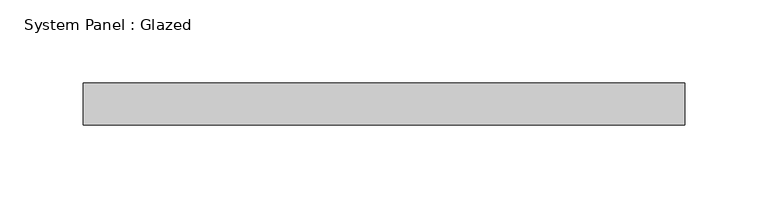
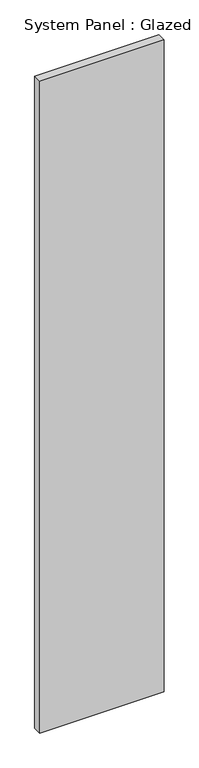
"""IFC4 building model written with IfcOpenShell, lengths in millimetres: plate geometry, System Panel : Glazed."""

from ifc_helpers import new_model, si_unit, origin, origin_with_axes, place, context, project, spatial, polyline, outline, extrude, source, transform, mapped, element, save


def system_panel_glazed_935821d8(model_context):
    return source(origin(), model_context, "Body", "SweptSolid", [
        extrude(outline(polyline([(180.975, 19.05), (-180.975, 19.05), (-180.975, 44.45), (180.975, 44.45), (180.975, 19.05)])), origin_with_axes(), (0.0, 0.0, 1.0), 2006.6),
    ])


if __name__ == "__main__":
    model = new_model("IFC4")
    model_context = context("Model", 3, world=origin())
    ifc_project = project(units=[si_unit("LENGTHUNIT", "METRE", prefix="MILLI")], contexts=[model_context])
    site = spatial("IfcSite", under=ifc_project)
    building = spatial("IfcBuilding", under=site)
    placement = place(None, origin())
    system_panel_glazed_shape = system_panel_glazed_935821d8(model_context)
    element("IfcPlate", 1, ObjectType="System Panel : Glazed", at=placement, inside=building, context=model_context, shape_type="MappedRepresentation", body=[
        mapped(system_panel_glazed_shape, transform((0.0, 0.0, 0.0), x_axis=(1.0, 0.0, 0.0), y_axis=(0.0, 1.0, 0.0), z_axis=(0.0, 0.0, 1.0))),
    ])
    save(model, "model.ifc")

# Revit data of these elements
# Type "System Panel : Glazed"
#   Construction Type Id = "GSP4R"
#   Analytic Construction = "1/8 in Pilkington single glazing"
#   Visual Light Transmittance = 0.9
#   Solar Heat Gain Coefficient = 0.86
#   Heat Transfer Coefficient (U) = 1.18115 BTU/(h·ft²·°F)
#   Define Thermal Properties by = 1
# Element 1 (IfcPlate, "System Panel : Glazed")
#   Materials on its faces: "Glass"
# Materials
#   "Glass": class "Glass", colour RGB 0 128 192, transparency 0.75, Description = "Soda Lime Glass", Cost = 0
